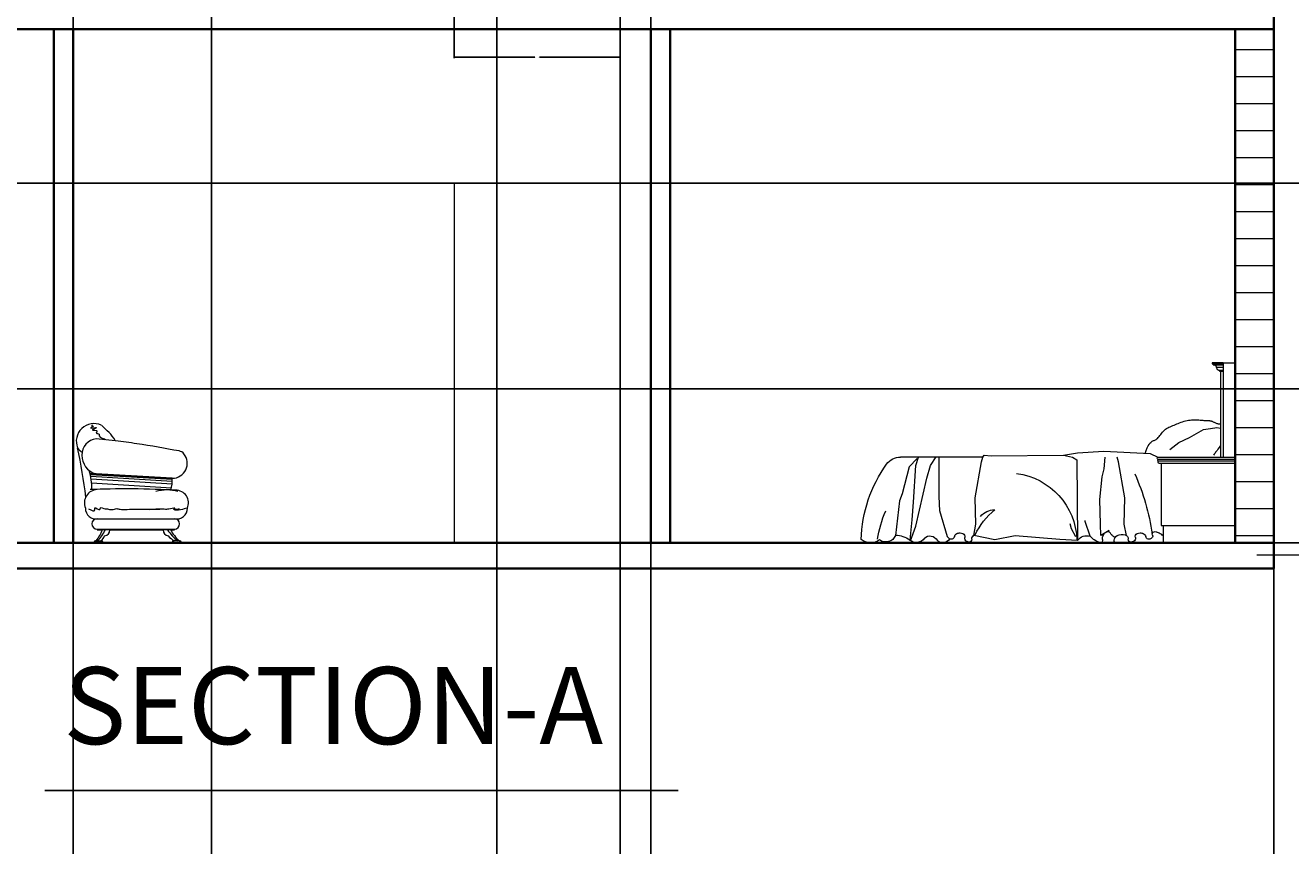
# Model space of a CAD drawing. Units: inches. Extents: x 1355 to 2746, y 1171 to 2751.
# Tile 21 of 24: x 2215 to 2510, y 2155 to 2346. Entities that reach past the tile are written whole.
import ezdxf

# ---------------------------------------------------------------- set-up
doc = ezdxf.new("R2010")
doc.units = ezdxf.units.IN
for name, color, linetype, lineweight in [('A-ANNO-DIMS', 2, 'Continuous', 18), ('A-ANNO-TEXT', 7, 'Continuous', 18), ('A-ANNO-TITL', 7, 'Continuous', 25), ('A-FURN', 8, 'Continuous', 13), ('A-SECT', 7, 'Continuous', 35), ('A-SECT-DOOR', 3, 'Continuous', 18), ('A-WALL-PATT', 252, 'Continuous', 13)]:
    doc.layers.add(name, color=color, linetype=linetype, lineweight=lineweight)
doc.styles.get("Standard").update_dxf_attribs({"font": 'arial.ttf'})
doc.dimstyles.get("Standard").update_dxf_attribs({"dimtxt": 0.18, "dimasz": 0.18, "dimexe": 0.18, "dimexo": 0.0625, "dimgap": 0.09, "dimtad": 0, "dimtih": 1, "dimtoh": 1, "dimdec": 4, "dimzin": 0, "dimdsep": 46, "dimtxsty": 'Standard', "dimcen": 0.09, "dimadec": 0, "dimazin": 0, "dimtfac": 1, "dimtdec": 4, "dimtofl": 0, "dimtmove": 0, "dimatfit": 3, "dimfxl": 1, "dimtolj": 1, "dimtzin": 0, "dimarcsym": 0})

# ---------------------------------------------------------------- blocks, each defined once
blk = doc.blocks.new('A$C2FF713C3')
for p, q in [((0, 1050.5), (0, 0.5)), ((70, 1050.5), (0, 1050.5)), ((70, 1050.5), (70, 500.5)), ((70, 1050.5), (133.7, 1050.5)), ((127.4, 1044.2), (70, 1044.2)), ((125.8, 1038), (70, 1038)), ((127.4, 1038), (125.8, 1038)), ((133.7, 1044.2), (127.4, 1044.2)), ((127.4, 1044.2), (127.4, 1038)), ((133.7, 1050.5), (133.7, 1044.2)), ((108.5, 1024.2), (70, 1024.2)), ((91.3, 1006.7), (70, 1006.7)), ((91.3, 1000.5), (70, 1000.5)), ((85, 1000.5), (85, 500.5)), ((97.5, 1006.7), (91.3, 1006.7)), ((91.3, 1006.7), (91.3, 1000.5)), ((87.4, 693.2), (83.6, 693.1)), ((107.4, 672.2), (85.3, 669.2)), ((91.2, 693.6), (87.4, 693.2)), ((95.1, 694.2), (91.2, 693.6)), ((99, 694.9), (95.1, 694.2)), ((102.9, 695.9), (99, 694.9)), ((106.8, 697), (102.9, 695.9)), ((110.7, 698.3), (106.8, 697)), ((144.4, 667.7), (107.4, 672.2)), ((114.5, 699.7), (110.7, 698.3)), ((118.2, 701.2), (114.5, 699.7)), ((121.8, 702.9), (118.2, 701.2)), ((125.3, 704.5), (121.8, 702.9)), ((128.7, 706.1), (125.3, 704.5)), ((131.9, 707.6), (128.7, 706.1)), ((134.9, 709), (131.9, 707.6)), ((137.8, 710.2), (134.9, 709)), ((140.5, 711.1), (137.8, 710.2)), ((143, 711.8), (140.5, 711.1)), ((145.5, 712.2), (143, 711.8)), ((184.4, 660.3), (144.4, 667.7)), ((148, 712.5), (145.5, 712.2)), ((150.6, 712.6), (148, 712.5)), ((153.6, 712.7), (150.6, 712.6)), ((156.9, 712.7), (153.6, 712.7)), ((160.7, 712.8), (156.9, 712.7)), ((165.1, 713), (160.7, 712.8)), ((170.2, 713.4), (165.1, 713)), ((175.9, 713.9), (170.2, 713.4)), ((182.3, 714.4), (175.9, 713.9)), ((189.2, 715), (182.3, 714.4)), ((196.5, 715.6), (189.2, 715)), ((204.1, 716.2), (196.5, 715.6)), ((212.1, 716.7), (204.1, 716.2)), ((220.3, 717.1), (212.1, 716.7)), ((228.7, 717.3), (220.3, 717.1)), ((237.2, 717.3), (228.7, 717.3)), ((245.8, 717.1), (237.2, 717.3)), ((254.4, 716.7), (245.8, 717.1)), ((263.2, 715.9), (254.4, 716.7)), ((271.9, 714.8), (263.2, 715.9)), ((280.7, 713.3), (271.9, 714.8)), ((289.5, 711.4), (280.7, 713.3)), ((298.2, 709.1), (289.5, 711.4)), ((306.9, 706.4), (298.2, 709.1)), ((315.5, 703.4), (306.9, 706.4)), ((324, 700.1), (315.5, 703.4)), ((332.3, 696.8), (324, 700.1)), ((340.6, 693.4), (332.3, 696.8)), ((348.7, 690), (340.6, 693.4)), ((356.6, 686.7), (348.7, 690)), ((364.3, 683.5), (356.6, 686.7)), ((371.9, 680.4), (364.3, 683.5)), ((379.2, 677.3), (371.9, 680.4)), ((386.3, 674), (379.2, 677.3)), ((393.1, 670.5), (386.3, 674)), ((399.8, 666.5), (393.1, 670.5)), ((406.2, 662.1), (399.8, 666.5)), ((267.2, 614.5), (184.4, 660.3)), ((327.9, 585), (267.2, 614.5)), ((412.3, 657), (406.2, 662.1)), ((418.1, 651.3), (412.3, 657)), ((423.7, 645.1), (418.1, 651.3)), ((429.1, 638.6), (423.7, 645.1)), ((434.2, 632), (429.1, 638.6)), ((439, 625.6), (434.2, 632)), ((443.7, 619.6), (439, 625.6)), ((448.1, 614.1), (443.7, 619.6)), ((452.4, 609.5), (448.1, 614.1)), ((456.4, 605.9), (452.4, 609.5)), ((460.3, 603), (456.4, 605.9)), ((464.2, 600.8), (460.3, 603)), ((468, 599.1), (464.2, 600.8)), ((471.7, 597.6), (468, 599.1)), ((475.6, 596.1), (471.7, 597.6)), ((479.6, 594.4), (475.6, 596.1)), ((483.7, 592.3), (479.6, 594.4)), ((488, 589.7), (483.7, 592.3)), ((84.9, 568), (93.7, 555.7)), ((93.7, 555.7), (100.6, 546.3)), ((100.6, 546.3), (105.9, 539)), ((105.9, 539), (110.1, 533.2)), ((110.1, 533.2), (113.9, 528.2)), ((113.9, 528.2), (117.6, 523.3)), ((117.6, 523.3), (121.8, 517.9)), ((121.8, 517.9), (127, 511.4)), ((381.3, 544.7), (327.9, 585)), ((495.7, 521.8), (450, 500.5)), ((492.6, 586), (488, 589.7)), ((497.4, 581), (492.6, 586)), ((766.6, 534.5), (495.7, 521.8)), ((502.4, 574.2), (497.4, 581)), ((507.8, 565.1), (502.4, 574.2)), ((513.4, 553.5), (507.8, 565.1)), ((519.3, 538.8), (513.4, 553.5)), ((525.6, 520.7), (519.3, 538.8)), ((919.2, 526), (766.6, 534.5)), ((1001, 512.1), (919.2, 526)), ((450, 500.5), (0, 500.5)), ((450, 488.5), (0, 488.5)), ((448.7, 477.5), (0, 477.5)), ((446.9, 465.5), (0, 465.5)), ((431.9, 465.5), (431.9, 100.5)), ((642.6, 263.3), (679.4, 472.9)), ((679.4, 472.9), (687.3, 500.5)), ((764.1, 432.4), (757.6, 500.5)), ((923, 485), (919.8, 13.9)), ((947.7, 499.8), (923, 485)), ((1001, 512.1), (947.7, 499.8)), ((1422.2, 508), (1001, 512.1)), ((1463.2, 511.6), (1422.2, 508)), ((1471.1, 500.5), (1463.2, 511.6)), ((1479, 472.9), (1471.1, 500.5)), ((1471.1, 500.5), (1951, 500.5)), ((1515.8, 263.3), (1479, 472.9)), ((1725.7, 369.9), (1725.7, 500.5)), ((1776.6, 450.8), (1743.5, 502.3)), ((1798.7, 377.3), (1776.6, 450.8)), ((1861.3, 450.8), (1846, 500.5)), ((1853.9, 491.3), (1901.8, 443.5)), ((1876, 237.5), (1861.3, 450.8)), ((1901.8, 443.5), (1942.3, 285.3)), ((775.1, 384.6), (764.1, 432.4)), ((789.8, 252.2), (775.1, 384.6)), ((1725.7, 270.6), (1725.7, 369.9)), ((1861.3, 97.8), (1798.7, 377.3)), ((646.3, 108.8), (642.6, 263.3)), ((786.1, 108.8), (789.8, 252.2)), ((1512.2, 108.8), (1515.8, 263.3)), ((1722, 186), (1725.7, 270.6)), ((1883.4, 134.6), (1876, 237.5)), ((1942.3, 285.3), (1957, 244.9)), ((1957, 244.9), (1981.3, 42.2)), ((1677.5, 36.3), (1722, 186)), ((431.9, 100.5), (0, 100.5)), ((419.9, 100.5), (419.9, 0.5)), ((634, 43.7), (646.3, 108.8)), ((782.5, 42.6), (786.1, 108.8)), ((844.9, 39.6), (874.4, 124.2)), ((874.4, 124.2), (875.1, 130)), ((956.4, 83.1), (931.8, 36.9)), ((964.4, 113.4), (956.4, 83.1)), ((1524.4, 43.7), (1512.2, 108.8)), ((1892.4, 12.1), (1861.3, 97.8)), ((1890.7, 57.3), (1883.4, 134.6)), ((0, 0.5), (419.9, 0.5)), ((734.6, 72), (782.5, 42.6)), ((919.8, 13.9), (1021.5, 19.4)), ((1021.5, 19.4), (1282.6, 41.6)), ((1282.6, 41.6), (1401.6, 17.8)), ((1401.6, 17.8), (1524.4, 43.7)), ((1894.7, 13.8), (1890.7, 57.3))]:
    blk.add_line(p, q)
for centre, radius, start, end in [((125, 1021.3), 16.8, 87.42116, 169.92904), ((90, 1023.7), 18.5, 293.7928, 1.50079), ((435.7, 473.3), 13.6, 324.97742, 17.95445), ((443.2, 483.7), 8.28, 310.99411, 35.0512), ((447.3, 494.5), 6.6, 294.61118, 65.38882), ((1951, 400.5), 100, 35.83195, 90), ((1396.7, 0.2), 783.8, 1.45705, 35.83195), ((1735.3, -117.1), 1261.8, 155.69024, 172.29016), ((1327.7, 3.6), 404.9, 97.57237, 178.02017), ((1400.1, 81.1), 112.5, 40.70885, 88.9264), ((1125.8, -139.2), 432.6, 25.56932, 50.29378), ((1449, -72.7), 642.9, 8.37443, 23.73381), ((259.9, 249), 261.9, 307.63119, 310.56693), ((478.1, -13.1), 79.2, 115.93806, 127.15402), ((517.4, -93.9), 169, 111.78143, 115.93806), ((474.5, 13.6), 53.3, 104.37799, 111.78143), ((466.1, 46.3), 19.5, 71.58245, 104.37799), ((464.6, 41.9), 24.2, 42.22901, 71.58245), ((490.7, 39.5), 10.2, 140.3102, 217.27929), ((475.7, 51.9), 9.23, 320.3102, 42.22901), ((513.6, 57), 39, 217.27929, 233.1579), ((500.7, 39.8), 17.5, 233.1579, 256.94088), ((500.6, 39.4), 17.2, 256.94088, 270), ((500.6, 74), 51.8, 270, 277.51528), ((505.3, 38.6), 16, 277.51528, 349.78267), ((546.4, 31.2), 25.7, 114.29273, 169.78267), ((554.4, 13.4), 45.2, 90, 114.29273), ((554.4, 20.7), 37.9, 63.42724, 90), ((562.2, 36.4), 20.3, 346.09021, 63.42724), ((601.7, 26.6), 20.3, 166.09021, 243.58133), ((609.7, 42.8), 38.3, 243.58133, 251.5824), ((612.4, 50.9), 46.9, 251.5824, 258.81111), ((606.5, 21.1), 16.5, 258.81111, 1.75785), ((648.9, 22.4), 25.9, 104.59371, 181.75785), ((658.8, -15.6), 65.2, 63.45814, 104.59371), ((673, 12.8), 33.4, 4.66977, 63.45814), ((674.1, 83.9), 58.7, 296.89415, 314.45228), ((713.3, 7.3), 7.4, 170.64836, 198.63453), ((677.4, 13.2), 29, 350.64836, 4.66977), ((711.6, 6.7), 5.58, 198.63453, 218.42959), ((207.6, 559.5), 724.9, 314.45228, 314.97091), ((575.9, 190.8), 203.8, 314.97091, 315.94905), ((696.8, 73.9), 35.6, 315.94905, 329.81727), ((762.4, 35.7), 40.4, 136.79901, 149.81727), ((740.9, 55.9), 10.9, 81.87802, 136.79901), ((738.1, 36.1), 30.8, 50.07733, 81.87802), ((735.6, 33.1), 34.7, 33.71681, 50.07733), ((690, 2.7), 89.5, 23.5428, 33.71681), ((747.6, 27.8), 26.6, 343.69737, 23.5428), ((788.5, 15.9), 15.9, 163.69737, 216.05798), ((783.9, 12.5), 10.2, 216.05798, 282.98191), ((759.3, 118.9), 119.4, 282.98191, 301.5385), ((783.2, 80.1), 73.8, 301.5385, 318.3377), ((782.8, 80.4), 74.3, 318.3377, 326.7067), ((863.8, -27), 69.2, 36.67542, 105.79154), ((957.7, 57), 57.3, 227.99499, 228.65775), ((1509.5, 22.4), 25.9, 358.24215, 61.16814), ((1551.9, 21.1), 16.5, 178.24215, 281.18889), ((1546, 50.9), 46.9, 281.18889, 288.4176), ((1548.7, 42.8), 38.3, 288.4176, 296.41867), ((1556.8, 26.6), 20.3, 296.41867, 13.90979), ((1596.2, 36.4), 20.3, 116.57276, 193.90979), ((1604, 20.7), 37.9, 90, 116.57276), ((1604, 13.4), 45.2, 65.70727, 90), ((1612, 31.2), 25.7, 10.21733, 65.70727), ((1653.1, 38.6), 16, 190.21733, 262.48472), ((1657.8, 74), 51.8, 262.48472, 270), ((1657.8, 39.4), 17.2, 270, 283.05912), ((1657.7, 39.8), 17.5, 283.05912, 306.8421), ((1704.6, 43.4), 43.5, 208.05971, 320.53056), ((1644.8, 57), 39, 306.8421, 322.72071), ((1667.7, 39.5), 10.2, 322.72071, 344.91412), ((1779.5, -6.4), 46.9, 46.72075, 151.78128), ((1859.7, 59.2), 57.3, 213.23769, 312.00501), ((1983.6, -94.9), 140.5, 91.35454, 127.50961), ((2036.9, 65.4), 60.1, 201.78863, 308.33048), ((2126, 84.9), 84.4, 232.07783, 309.92484)]:
    blk.add_arc(centre, radius, start, end)
blk = doc.blocks.new('A$C28ED0BDC')
for p, q in [((300.7, 778.6), (176.5, 792.9)), ((737.6, 490.8), (105.1, 529.1)), ((737.6, 485.8), (106.3, 524)), ((737.6, 480.8), (107.5, 518.9)), ((737.5, 465.8), (110.8, 503.7)), ((735.8, 445.9), (114.2, 483.5)), ((730.6, 416.3), (117.6, 453.3)), ((158.9, 100), (753.7, 100)), ((158.9, 100), (158.9, 95)), ((169.3, 180), (753.7, 180)), ((753.7, 100), (753.7, 95)), ((204.4, 0), (136.7, 0)), ((151.7, 10), (146, 10)), ((151.7, 10), (189.4, 10)), ((158.9, 95), (200.3, 95)), ((195, 10), (189.4, 10)), ((195, 10), (189.4, 10)), ((257.3, 95), (200.3, 95)), ((257.3, 95), (666.7, 95)), ((723.7, 95), (666.7, 95)), ((723.7, 95), (753.7, 95)), ((737.8, 0), (805.4, 0)), ((747.1, 10), (752.8, 10)), ((747.1, 10), (752.8, 10)), ((790.4, 10), (752.8, 10)), ((790.4, 10), (796.1, 10))]:
    blk.add_line(p, q)
for centre, radius, start, end in [((135.3, 776.3), 135.9, 65.3492, 202.21563), ((162.8, 673.6), 120, 83.43842, 170.98936), ((-3552.4, -58.3), 3647.1, 6.37823, 12.40155), ((93.2, 779.5), 99.8, 213.09621, 240.68048), ((193.2, 668.8), 150.8, 170.98936, 243.39142), ((780.2, 642.1), 60, 37.32442, 79.59851), ((737, 606.7), 115.8, 270.2622, 38.33495), ((-328, 418.8), 446.9, 358.17507, 17.23744), ((179.4, 641.3), 120, 243.39142, 252.67687), ((458.5, 479.3), 279.3, 343.50497, 2.36848), ((164.5, 301.2), 103.1, 93.095, 202.35798), ((696.5, 85.3), 315.8, 74.36238, 105.63762), ((763.8, 301.7), 98.3, 336.20857, 89.98148), ((151.5, 260.4), 82.4, 178.89673, 282.44534), ((771.4, 260.4), 82.4, 257.55466, 1.10327), ((158.9, 140), 40, 90, 270), ((753.7, 140), 40, 270, 90), ((148.9, -2), 12.3, 103.33506, 170.71519), ((-63.8, 189.5), 280.5, 320.20721, 340.30535), ((-29.3, 210.6), 277.5, 313.71744, 335.39036), ((124.1, 86.8), 100.8, 310.34673, 337.03101), ((192.2, -2), 12.3, 9.28481, 76.66494), ((210.9, 93.5), 46.4, 277.43329, 1.84553), ((713.1, 93.5), 46.4, 178.15447, 262.56671), ((987.3, 281.2), 341.5, 213.0378, 232.56776), ((831, 152.1), 162.1, 220.15958, 241.18286), ((1022.2, 260.8), 341.5, 209.04881, 227.25949), ((750, -2), 12.3, 103.33506, 170.71519), ((793.3, -2), 12.3, 9.28481, 76.66494)]:
    blk.add_arc(centre, radius, start, end)
for points, knots in [([(123.9, 901.3), (120.7, 897.9), (113.5, 890.1), (146.7, 895.3), (73.3, 866.1), (197.2, 892.5), (86.1, 854.7), (175.1, 866.1), (141.9, 832.2), (182.3, 838), (163.3, 800.3), (225.2, 796.2), (219.8, 787.9)], [0, 0, 0, 0, 9.765075, 22.239713, 47.817951, 93.447543, 130.976544, 169.416587, 185.180341, 209.428428, 221.888603, 276.469797, 276.469797, 276.469797, 276.469797]), ([(300.7, 778.6), (300.1, 779.6), (269.8, 832.3), (237.8, 855.2), (192, 899.8)], [244.920573, 244.920573, 244.920573, 244.920573, 247.928636, 395.738949, 395.738949, 395.738949, 395.738949]), ([(791, 701.1), (682.8, 721), (519.9, 750.6), (355.8, 771.9), (300.7, 778.6)], [18.761969, 18.761969, 18.761969, 18.761969, 348.756072, 515.290542, 515.290542, 515.290542, 515.290542]), ([(763.8, 400), (674.2, 404.2), (398.1, 413.1), (207.8, 407.5), (107.2, 404.2)], [0, 0, 0, 0, 269.198238, 571.026582, 571.026582, 571.026582, 571.026582]), ([(93.5, 256.7), (117.3, 244.2), (148.3, 227.9), (135.5, 280.6), (184.2, 233.2), (182.4, 277.4), (213.7, 254), (239, 258.5), (267.4, 245.2), (313.7, 262.9), (325.5, 247.1), (418.5, 255), (547.8, 252.8), (616.1, 255.7), (660.2, 256.5)], [0, 0, 0, 0, 49.407579, 64.565784, 105.844847, 118.345477, 155.269185, 167.410003, 198.361737, 241.285001, 308.128282, 447.747709, 520.592639, 652.828768, 652.828768, 652.828768, 652.828768]), ([(848.7, 261.5), (836.7, 257.2), (814, 248.9), (727, 241.4), (826.7, 263.1), (729.9, 243.1), (771.4, 265.6), (713.2, 252.2), (686.6, 252.2), (629, 252.7), (589.5, 250.5), (564.7, 249.2)], [0, 0, 0, 0, 49.380651, 92.855981, 126.791693, 168.915675, 179.762432, 213.696461, 251.182, 296.320949, 372.653556, 372.653556, 372.653556, 372.653556])]:
    blk.add_open_spline(points, degree=3, knots=knots)
blk = doc.blocks.new('DOOR-OPENING-SECTION')
for p, q in [((0, 84), (0, 0)), ((38.81, 84), (0, 84)), ((38.81, 84), (38.81, 0))]:
    blk.add_line(p, q)
blk = doc.blocks.new('*D94')
at = {"layer": 'A-ANNO-DIMS', "color": 0, "lineweight": -2, "transparency": 16777216}
for p, q in [((2314.9, 2351.34), (2314.9, 2338.62)), ((2353.71, 2351.34), (2353.71, 2338.62)), ((2315.08, 2338.8), (2333.78, 2338.8)), ((2353.53, 2338.8), (2334.83, 2338.8))]:
    blk.add_line(p, q, dxfattribs=at)
at = {"layer": 'A-ANNO-DIMS', "color": 0, "transparency": 16777216}
for points in [[(2315.08, 2338.83), (2315.08, 2338.77), (2314.9, 2338.8)], [(2353.53, 2338.83), (2353.53, 2338.77), (2353.71, 2338.8)]]:
    blk.add_solid(points, dxfattribs=at)
at = {"layer": 'Defpoints', "color": 0, "transparency": 16777216}
for p in [(2314.9, 2351.4), (2353.71, 2351.4), (2353.71, 2338.8)]:
    blk.add_point(p, dxfattribs=at)
at = {"layer": 'A-ANNO-DIMS', "color": 0, "transparency": 16777216, "insert": (2334.31, 2338.8), "char_height": 0.18, "attachment_point": 5}
blk.add_mtext('\\A1;39 TYP.', dxfattribs=at)
blk = doc.blocks.new('*D99')
at = {"layer": 'A-ANNO-DIMS', "color": 0, "lineweight": -2, "transparency": 16777216}
for p, q in [((2080.39, 2139.36), (2080.39, 2716.58)), ((2080.57, 2716.4), (2152.75, 2716.4)), ((2225.71, 2716.4), (2153.53, 2716.4)), ((2225.89, 2139.36), (2225.89, 2716.58))]:
    blk.add_line(p, q, dxfattribs=at)
at = {"layer": 'A-ANNO-DIMS', "color": 0, "transparency": 16777216}
for points in [[(2080.57, 2716.43), (2080.57, 2716.37), (2080.39, 2716.4)], [(2225.71, 2716.43), (2225.71, 2716.37), (2225.89, 2716.4)]]:
    blk.add_solid(points, dxfattribs=at)
at = {"layer": 'Defpoints', "color": 0, "transparency": 16777216}
for p in [(2225.89, 2716.4), (2080.39, 2139.3), (2225.89, 2139.3)]:
    blk.add_point(p, dxfattribs=at)
at = {"layer": 'A-ANNO-DIMS', "color": 0, "transparency": 16777216, "insert": (2153.14, 2716.4), "char_height": 0.18, "attachment_point": 5}
blk.add_mtext('\\A1;145.5', dxfattribs=at)
blk = doc.blocks.new('*D100')
at = {"layer": 'A-ANNO-DIMS', "color": 0, "lineweight": -2, "transparency": 16777216}
for p, q in [((2225.89, 2139.36), (2225.89, 2716.58)), ((2226.07, 2716.4), (2293.11, 2716.4)), ((2360.71, 2716.4), (2293.67, 2716.4)), ((2360.89, 2139.36), (2360.89, 2716.58))]:
    blk.add_line(p, q, dxfattribs=at)
at = {"layer": 'A-ANNO-DIMS', "color": 0, "transparency": 16777216}
for points in [[(2226.07, 2716.43), (2226.07, 2716.37), (2225.89, 2716.4)], [(2360.71, 2716.43), (2360.71, 2716.37), (2360.89, 2716.4)]]:
    blk.add_solid(points, dxfattribs=at)
at = {"layer": 'Defpoints', "color": 0, "transparency": 16777216}
for p in [(2360.89, 2716.4), (2225.89, 2139.3), (2360.89, 2139.3)]:
    blk.add_point(p, dxfattribs=at)
at = {"layer": 'A-ANNO-DIMS', "color": 0, "transparency": 16777216, "insert": (2293.39, 2716.4), "char_height": 0.18, "attachment_point": 5}
blk.add_mtext('\\A1;135', dxfattribs=at)
blk = doc.blocks.new('*D101')
at = {"layer": 'A-ANNO-DIMS', "color": 0, "lineweight": -2, "transparency": 16777216}
for p, q in [((2360.89, 2139.36), (2360.89, 2716.58)), ((2361.07, 2716.4), (2433.25, 2716.4)), ((2506.21, 2716.4), (2434.03, 2716.4)), ((2506.39, 2139.36), (2506.39, 2716.58))]:
    blk.add_line(p, q, dxfattribs=at)
at = {"layer": 'A-ANNO-DIMS', "color": 0, "transparency": 16777216}
for points in [[(2361.07, 2716.43), (2361.07, 2716.37), (2360.89, 2716.4)], [(2506.21, 2716.43), (2506.21, 2716.37), (2506.39, 2716.4)]]:
    blk.add_solid(points, dxfattribs=at)
at = {"layer": 'Defpoints', "color": 0, "transparency": 16777216}
for p in [(2506.39, 2716.4), (2360.89, 2139.3), (2506.39, 2139.3)]:
    blk.add_point(p, dxfattribs=at)
at = {"layer": 'A-ANNO-DIMS', "color": 0, "transparency": 16777216, "insert": (2433.64, 2716.4), "char_height": 0.18, "attachment_point": 5}
blk.add_mtext('\\A1;145.5', dxfattribs=at)
blk = doc.blocks.new('*D112')
at = {"layer": 'A-ANNO-DIMS', "color": 0, "lineweight": -2, "transparency": 16777216}
for p, q in [((2258.27, 2095.29), (2258.27, 2716.58)), ((2258.45, 2716.4), (2291.19, 2716.4)), ((2324.72, 2716.4), (2291.98, 2716.4)), ((2324.9, 2095.29), (2324.9, 2716.58))]:
    blk.add_line(p, q, dxfattribs=at)
at = {"layer": 'A-ANNO-DIMS', "color": 0, "transparency": 16777216}
for points in [[(2258.45, 2716.43), (2258.45, 2716.37), (2258.27, 2716.4)], [(2324.72, 2716.43), (2324.72, 2716.37), (2324.9, 2716.4)]]:
    blk.add_solid(points, dxfattribs=at)
at = {"layer": 'Defpoints', "color": 0, "transparency": 16777216}
for p in [(2324.9, 2716.4), (2258.27, 2095.22), (2324.9, 2095.22)]:
    blk.add_point(p, dxfattribs=at)
at = {"layer": 'A-ANNO-DIMS', "color": 0, "transparency": 16777216, "insert": (2291.58, 2716.4), "char_height": 0.18, "attachment_point": 5}
blk.add_mtext('\\A1;66.63', dxfattribs=at)
blk = doc.blocks.new('*D123')
at = {"layer": 'A-ANNO-DIMS', "color": 0, "lineweight": -2, "transparency": 16777216}
for p, q in [((1880.77, 2261.4), (2648.07, 2261.4)), ((2647.89, 2261.22), (2647.89, 2243.58)), ((2647.89, 2225.58), (2647.89, 2243.22)), ((1940.77, 2225.4), (2648.07, 2225.4))]:
    blk.add_line(p, q, dxfattribs=at)
at = {"layer": 'A-ANNO-DIMS', "color": 0, "transparency": 16777216}
for points in [[(2647.86, 2261.22), (2647.92, 2261.22), (2647.89, 2261.4)], [(2647.86, 2225.58), (2647.92, 2225.58), (2647.89, 2225.4)]]:
    blk.add_solid(points, dxfattribs=at)
at = {"layer": 'Defpoints', "color": 0, "transparency": 16777216}
for p in [(1880.71, 2261.4), (2647.89, 2261.4), (1940.71, 2225.4)]:
    blk.add_point(p, dxfattribs=at)
at = {"layer": 'A-ANNO-DIMS', "color": 0, "transparency": 16777216, "insert": (2647.89, 2243.4), "char_height": 0.18, "attachment_point": 5}
blk.add_mtext('\\A1;36', dxfattribs=at)
blk = doc.blocks.new('*D125')
at = {"layer": 'A-ANNO-DIMS', "color": 0, "lineweight": -2, "transparency": 16777216}
for p, q in [((1880.77, 2309.4), (2648.07, 2309.4)), ((2647.89, 2309.22), (2647.89, 2285.58)), ((2647.89, 2261.58), (2647.89, 2285.22)), ((1880.77, 2261.4), (2648.07, 2261.4))]:
    blk.add_line(p, q, dxfattribs=at)
at = {"layer": 'A-ANNO-DIMS', "color": 0, "transparency": 16777216}
for points in [[(2647.86, 2309.22), (2647.92, 2309.22), (2647.89, 2309.4)], [(2647.86, 2261.58), (2647.92, 2261.58), (2647.89, 2261.4)]]:
    blk.add_solid(points, dxfattribs=at)
at = {"layer": 'Defpoints', "color": 0, "transparency": 16777216}
for p in [(1880.71, 2309.4), (2647.89, 2309.4), (1880.71, 2261.4)]:
    blk.add_point(p, dxfattribs=at)
at = {"layer": 'A-ANNO-DIMS', "color": 0, "transparency": 16777216, "insert": (2647.89, 2285.4), "char_height": 0.18, "attachment_point": 5}
blk.add_mtext('\\A1;48', dxfattribs=at)
blk = doc.blocks.new('*D126')
at = {"layer": 'A-ANNO-DIMS', "color": 0, "lineweight": -2, "transparency": 16777216}
for p, q in [((2080.39, 2219.34), (2080.39, 1171.06)), ((2506.39, 2219.34), (2506.39, 1171.06)), ((2080.57, 1171.24), (2293.1, 1171.24)), ((2506.21, 1171.24), (2293.68, 1171.24))]:
    blk.add_line(p, q, dxfattribs=at)
at = {"layer": 'A-ANNO-DIMS', "color": 0, "transparency": 16777216}
for points in [[(2080.57, 1171.27), (2080.57, 1171.21), (2080.39, 1171.24)], [(2506.21, 1171.27), (2506.21, 1171.21), (2506.39, 1171.24)]]:
    blk.add_solid(points, dxfattribs=at)
at = {"layer": 'Defpoints', "color": 0, "transparency": 16777216}
for p in [(2080.39, 2219.4), (2506.39, 2219.4), (2506.39, 1171.24)]:
    blk.add_point(p, dxfattribs=at)
at = {"layer": 'A-ANNO-DIMS', "color": 0, "transparency": 16777216, "insert": (2293.39, 1171.24), "char_height": 0.18, "attachment_point": 5}
blk.add_mtext('\\A1;426', dxfattribs=at)
blk = doc.blocks.new('*D134')
at = {"layer": 'A-ANNO-DIMS', "color": 0, "lineweight": -2, "transparency": 16777216}
for p, q in [((2353.71, 2477.34), (2353.71, 1171.06)), ((2360.89, 2477.34), (2360.89, 1171.06)), ((2353.89, 1171.24), (2356.92, 1171.24)), ((2360.71, 1171.24), (2357.68, 1171.24))]:
    blk.add_line(p, q, dxfattribs=at)
at = {"layer": 'A-ANNO-DIMS', "color": 0, "transparency": 16777216}
for points in [[(2353.89, 1171.27), (2353.89, 1171.21), (2353.71, 1171.24)], [(2360.71, 1171.27), (2360.71, 1171.21), (2360.89, 1171.24)]]:
    blk.add_solid(points, dxfattribs=at)
at = {"layer": 'Defpoints', "color": 0, "transparency": 16777216}
for p in [(2353.71, 2477.4), (2360.89, 2477.4), (2360.89, 1171.24)]:
    blk.add_point(p, dxfattribs=at)
at = {"layer": 'A-ANNO-DIMS', "color": 0, "transparency": 16777216, "insert": (2357.3, 1171.24), "char_height": 0.18, "attachment_point": 5}
blk.add_mtext('\\A1;7.181', dxfattribs=at)

msp = doc.modelspace()

# ---------------------------------------------------------------- hatches: boundary and pattern name
at = {"layer": 'A-WALL-PATT'}
h = msp.add_hatch(dxfattribs=at)
h.set_pattern_fill('ANSI32', color=256)
h.paths.add_polyline_path([(1660.2083, 2139.3018), (1614.5977, 2139.3018), (1614.5977, 2130.3018), (1655.7083, 2130.3018), (1655.7083, 1981.8018), (1660.2083, 1981.8018), (1660.2083, 2090.7225), (1692.5832, 2090.7225), (1692.5832, 2095.2225), (1660.2083, 2095.2225)])
h.paths.add_polyline_path([(1523.7083, 2130.3018), (1554.5977, 2130.3018), (1554.5977, 2134.8018), (1554.5977, 2139.3018), (1514.7083, 2139.3018), (1514.7083, 2071.8385), (1523.7083, 2071.8385)])
h.paths.add_polyline_path([(1940.7083, 2139.3018), (1883.7928, 2139.3018), (1883.7928, 2130.3018), (1931.7083, 2130.3018), (1931.7083, 2098.3333), (1940.7083, 2098.3333)])
h.paths.add_polyline_path([(1799.7083, 2130.3018), (1823.7928, 2130.3018), (1823.7928, 2134.8018), (1823.7928, 2139.3018), (1795.2083, 2139.3018), (1795.2083, 2130.3018), (1795.2083, 2095.2225), (1759.2134, 2095.2225), (1759.2134, 2090.7225), (1795.2083, 2090.7225), (1795.2083, 1981.8018), (1799.7083, 1981.8018), (1799.7083, 1986.3018)])
h.paths.add_polyline_path([(1940.7083, 2038.3333), (1931.7083, 2038.3333), (1931.7083, 1986.3018), (1832.7083, 1986.3018), (1832.7083, 1947.1338), (1837.2083, 1947.1338), (1837.2083, 1981.8018), (1931.7083, 1981.8018), (1931.7083, 1967.1939), (1940.7083, 1967.1939)])
h.paths.add_polyline_path([(1940.7083, 1943.1939), (1931.7083, 1943.1939), (1931.7083, 1921.8018), (1837.2083, 1921.8018), (1837.2083, 1926.0511), (1832.7083, 1926.0511), (1832.7083, 1917.3018), (1931.7083, 1917.3018), (1931.7083, 1908.3321), (1940.7083, 1908.3321)])
h.paths.add_polyline_path([(1940.7083, 1884.3321), (1931.7083, 1884.3321), (1931.7083, 1869.3018), (1899.4583, 1869.3018), (1899.4583, 1864.8018), (1931.7083, 1864.8018), (1931.7083, 1773.3018), (1786.5143, 1773.3018), (1786.5143, 1764.3018), (1844.7083, 1764.3018), (1844.7083, 1748.9343), (1853.7083, 1748.9343), (1853.7083, 1764.3018), (1931.7083, 1764.3018), (1931.7083, 1652.9424), (1940.7083, 1652.9424)])
h.paths.add_polyline_path([(1799.7083, 1864.8018), (1806.0522, 1864.8018), (1806.0522, 1867.0518), (1806.0522, 1869.3018), (1799.7083, 1869.3018), (1799.7083, 1917.3018), (1799.7083, 1921.8018), (1795.2083, 1921.8018), (1795.2083, 1773.3018), (1799.7083, 1773.3018)])
h.paths.add_polyline_path([(1872.8988, 1867.0518), (1872.8988, 1869.3018), (1867.2083, 1869.3018), (1867.2083, 1917.3018), (1862.7083, 1917.3018), (1862.7083, 1869.3018), (1836.9546, 1869.3018), (1836.9546, 1864.8018), (1862.7083, 1864.8018), (1872.8988, 1864.8018)])
h.paths.add_polyline_path([(1749.2197, 1773.3018), (1655.7083, 1773.3018), (1523.7083, 1773.3018), (1523.7083, 1828.4963), (1514.7083, 1828.4963), (1514.7083, 1753.9033), (1519.2083, 1753.9033), (1523.7083, 1753.9033), (1523.7083, 1764.3018), (1655.7083, 1764.3018), (1749.2197, 1764.3018), (1749.2197, 1768.8018)])
h.paths.add_polyline_path([(1660.2083, 1921.8018), (1655.7083, 1921.8018), (1655.7083, 1917.3018), (1655.7083, 1773.3018), (1660.2083, 1773.3018)])
h.paths.add_polyline_path([(1523.7083, 2011.8385), (1514.7083, 2011.8385), (1514.7083, 1973.114), (1519.2083, 1973.114), (1523.7083, 1973.114), (1523.7083, 1976.8227), (1523.7083, 1981.8018), (1618.2083, 1981.8018), (1618.2083, 1921.8018), (1553.707, 1921.8018), (1553.707, 1917.3018), (1622.7083, 1917.3018), (1622.7083, 1919.5518), (1622.7083, 1921.8018), (1622.7083, 1986.3018), (1523.7083, 1986.3018)])
h.paths.add_polyline_path([(1529.6686, 1919.5518), (1529.6686, 1921.8018), (1523.7083, 1921.8018), (1523.7083, 1949.114), (1514.7083, 1949.114), (1514.7083, 1888.4963), (1523.7083, 1888.4963), (1523.7083, 1917.3018), (1529.6686, 1917.3018)])
h.paths.add_polyline_path([(1538.9419, 1775.643), (1585.5504, 1775.643), (1585.5504, 1798.0318), (1538.9419, 1798.0318)], flags=25)
h.paths.add_polyline_path([(1696.7097, 1497.3356), (1769.5651, 1497.3356), (1769.5651, 1523.4559), (1696.7097, 1523.4559)], flags=9)
h.paths.add_polyline_path([(1629.1643, 1230.5133), (1877.0879, 1230.5133), (1877.0879, 1267.606), (1629.1643, 1267.606)], flags=9)
h.paths.add_polyline_path([(2533.4462, 2215.4033), (2579.9292, 2215.4033), (2579.9292, 2231.889), (2533.4462, 2231.889)], flags=9)
h.paths.add_polyline_path([(2540.822, 2515.6945), (2594.2245, 2515.6945), (2594.2245, 2545.5463), (2540.822, 2545.5463)], flags=9)
h.paths.add_polyline_path([(2535.9857, 2588.2819), (2582.4687, 2588.2819), (2582.4687, 2604.7675), (2535.9857, 2604.7675)], flags=9)
h.paths.add_polyline_path([(2537.1627, 2617.1172), (2649.1245, 2617.1172), (2649.1245, 2633.6029), (2537.1627, 2633.6029)], flags=9)
h.paths.add_polyline_path([(2218.0051, 2168.228), (2363.9573, 2168.228), (2363.9573, 2205.3208), (2218.0051, 2205.3208)], flags=9)
h.paths.add_polyline_path([(1650.2156, 2165.3631), (1800.3547, 2165.3631), (1800.3547, 2202.4559), (1650.2156, 2202.4559)], flags=9)
h.paths.add_polyline_path([(2553.9592, 1610.7663), (2588.4203, 1610.7663), (2588.4203, 1660.2233), (2553.9592, 1660.2233)], flags=9)
h.paths.add_polyline_path([(1549.0868, 1648.2033), (1595.6952, 1648.2033), (1595.6952, 1670.5921), (1549.0868, 1670.5921)], flags=9)
h.paths.add_polyline_path([(1546.9525, 1502.0931), (1583.3413, 1502.0931), (1583.3413, 1524.4819), (1546.9525, 1524.4819)], flags=9)
h.paths.add_polyline_path([(1540.7704, 1433.4431), (1587.3788, 1433.4431), (1587.3788, 1455.8319), (1540.7704, 1455.8319)], flags=9)
h.paths.add_polyline_path([(1683.6524, 1321.5269), (1760.6169, 1321.5269), (1760.6169, 1333.8911), (1683.6524, 1333.8911)], flags=9)
h.paths.add_polyline_path([(1832.0485, 1356.0874), (1873.0989, 1356.0874), (1873.0989, 1378.4762), (1832.0485, 1378.4762)], flags=9)
h.paths.add_polyline_path([(1877.9694, 1431.2138), (1926.3827, 1431.2138), (1926.3827, 1453.578), (1877.9694, 1453.578)], flags=9)
h.paths.add_polyline_path([(1847.3106, 1499.8371), (1883.6994, 1499.8371), (1883.6994, 1522.2259), (1847.3106, 1522.2259)], flags=9)
h.paths.add_polyline_path([(1813.7015, 1640.7287), (1860.3099, 1640.7287), (1860.3099, 1663.1175), (1813.7015, 1663.1175)], flags=9)
h.paths.add_polyline_path([(1876.2576, 1710.2471), (1912.9452, 1710.2471), (1912.9452, 1732.6359), (1876.2576, 1732.6359)], flags=25)
h.paths.add_polyline_path([(1695.9163, 1715.3064), (1736.9668, 1715.3064), (1736.9668, 1737.6952), (1695.9163, 1737.6952)], flags=9)
h.paths.add_polyline_path([(1881.8583, 1888.9094), (1930.2717, 1888.9094), (1930.2717, 1911.2737), (1881.8583, 1911.2737)], flags=9)
h.paths.add_polyline_path([(1823.9298, 1798.6431), (1864.9803, 1798.6431), (1864.9803, 1821.0319), (1823.9298, 1821.0319)], flags=25)
h.paths.add_polyline_path([(1845.6062, 1948.1408), (1881.995, 1948.1408), (1881.995, 1970.5296), (1845.6062, 1970.5296)], flags=25)
h.paths.add_polyline_path([(1849.027, 1991.5151), (1895.6355, 1991.5151), (1895.6355, 2013.9039), (1849.027, 2013.9039)], flags=25)
h.paths.add_polyline_path([(1684.9725, 2113.8416), (1764.2658, 2113.8416), (1764.2658, 2126.2058), (1684.9725, 2126.2058)], flags=9)
h.paths.add_polyline_path([(1688.6193, 1913.0676), (1776.2005, 1913.0676), (1776.2005, 1935.4564), (1688.6193, 1935.4564)], flags=9)
h.paths.add_polyline_path([(1571.4689, 1930.9816), (1607.8577, 1930.9816), (1607.8577, 1953.3704), (1571.4689, 1953.3704)], flags=25)
h.paths.add_polyline_path([(1535.3581, 1998.3125), (1581.9665, 1998.3125), (1581.9665, 2020.7014), (1535.3581, 2020.7014)], flags=9)
h = msp.add_hatch(dxfattribs=at)
h.set_pattern_fill('ANSI32', color=256)
h.paths.add_polyline_path([(1749.2197, 1686.3018), (1732.6892, 1686.3018), (1523.7083, 1686.3018), (1523.7083, 1705.9033), (1514.7083, 1705.9033), (1514.7083, 1647.8732), (1519.2083, 1647.8732), (1523.7083, 1647.8732), (1523.7083, 1677.3018), (1655.7083, 1677.3018), (1655.7083, 1528.8018), (1660.2083, 1528.8018), (1660.2083, 1677.3018), (1732.6892, 1677.3018), (1749.2197, 1677.3018)])
h.paths.add_polyline_path([(1931.7083, 1686.3018), (1853.7083, 1686.3018), (1853.7083, 1703.5696), (1844.7083, 1703.5696), (1844.7083, 1686.3018), (1788.0274, 1686.3018), (1788.0274, 1677.3018), (1795.2083, 1677.3018), (1795.2083, 1528.8018), (1799.7083, 1528.8018), (1799.7083, 1677.3018), (1844.7083, 1677.3018), (1931.7083, 1677.3018)])
h.paths.add_polyline_path([(1931.7083, 1533.3018), (1844.7083, 1533.3018), (1832.7083, 1533.3018), (1832.7083, 1531.0518), (1832.7083, 1528.8018), (1832.7083, 1495.7519), (1837.2083, 1495.7519), (1837.2083, 1528.8018), (1931.7083, 1528.8018)])
h.paths.add_polyline_path([(1940.7083, 1592.9424), (1931.7083, 1592.9424), (1931.7083, 1506.7845), (1940.7083, 1506.7845)])
h.paths.add_polyline_path([(1940.7083, 1482.7845), (1936.2083, 1482.7845), (1931.7083, 1482.7845), (1931.7083, 1320.3018), (1880.7083, 1320.3018), (1880.7083, 1311.3018), (1940.7083, 1311.3018)])
h.paths.add_polyline_path([(1931.7083, 1468.8018), (1844.7083, 1468.8018), (1837.2083, 1468.8018), (1837.2083, 1474.34), (1832.7083, 1474.34), (1832.7083, 1468.8018), (1832.7083, 1464.3018), (1844.7083, 1464.3018), (1931.7083, 1464.3018)])
h.paths.add_polyline_path([(1863.8571, 1464.3018), (1859.3571, 1464.3018), (1859.3571, 1404.1662), (1838.1542, 1404.1662), (1838.1542, 1399.8018), (1869.4185, 1399.8018), (1869.4185, 1402.0518), (1869.4185, 1404.3018), (1863.8571, 1404.3018)])
h.paths.add_polyline_path([(1799.7083, 1399.6662), (1805.4082, 1399.6662), (1805.4082, 1401.9162), (1805.4082, 1404.1662), (1799.7083, 1404.1662), (1799.7083, 1464.3018), (1799.7083, 1468.8018), (1795.2083, 1468.8018), (1795.2083, 1356.2098), (1761.2597, 1356.2098), (1761.2597, 1351.7098), (1795.2083, 1351.7098), (1795.2083, 1320.3018), (1795.2083, 1311.3018), (1844.7083, 1311.3018), (1844.7083, 1315.8018), (1844.7083, 1320.3018), (1799.7083, 1320.3018)])
h.paths.add_polyline_path([(1692.9218, 1356.2098), (1660.2083, 1356.2098), (1660.2083, 1430.786), (1657.9583, 1430.786), (1655.7083, 1430.786), (1655.7083, 1320.3018), (1611.934, 1320.3018), (1611.934, 1311.3018), (1660.2083, 1311.3018), (1660.2083, 1351.7098), (1692.9218, 1351.7098)])
h.paths.add_polyline_path([(1523.7083, 1372.653), (1514.7083, 1372.653), (1514.7083, 1311.3018), (1551.934, 1311.3018), (1551.934, 1315.8018), (1551.934, 1320.3018), (1523.7083, 1320.3018)])
h.paths.add_polyline_path([(1523.7083, 1490.9023), (1514.7083, 1490.9023), (1514.7083, 1432.653), (1519.2083, 1432.653), (1523.7083, 1432.653)])
h.paths.add_polyline_path([(1660.2083, 1468.8018), (1622.7083, 1468.8018), (1622.7083, 1473.1566), (1618.2083, 1473.1566), (1618.2083, 1468.8018), (1523.7083, 1468.8018), (1523.7083, 1464.3018), (1655.7083, 1464.3018), (1655.7083, 1460.5634), (1660.2083, 1460.5634)])
h.paths.add_polyline_path([(1523.7083, 1587.8732), (1514.7083, 1587.8732), (1514.7083, 1514.9023), (1519.2083, 1514.9023), (1523.7083, 1514.9023)])
h.paths.add_polyline_path([(1622.7083, 1533.3018), (1523.7083, 1533.3018), (1523.7083, 1528.8018), (1618.2083, 1528.8018), (1618.2083, 1494.4205), (1622.7083, 1494.4205), (1622.7083, 1528.8018)])
h.paths.add_polyline_path([(1696.7097, 1497.3356), (1769.5651, 1497.3356), (1769.5651, 1523.4559), (1696.7097, 1523.4559)], flags=9)
h.paths.add_polyline_path([(1629.1643, 1230.5133), (1877.0879, 1230.5133), (1877.0879, 1267.606), (1629.1643, 1267.606)], flags=9)
h.paths.add_polyline_path([(2533.4462, 2215.4033), (2579.9292, 2215.4033), (2579.9292, 2231.889), (2533.4462, 2231.889)], flags=9)
h.paths.add_polyline_path([(2540.822, 2515.6945), (2594.2245, 2515.6945), (2594.2245, 2545.5463), (2540.822, 2545.5463)], flags=9)
h.paths.add_polyline_path([(2535.9857, 2588.2819), (2582.4687, 2588.2819), (2582.4687, 2604.7675), (2535.9857, 2604.7675)], flags=9)
h.paths.add_polyline_path([(2537.1627, 2617.1172), (2649.1245, 2617.1172), (2649.1245, 2633.6029), (2537.1627, 2633.6029)], flags=9)
h.paths.add_polyline_path([(2218.0051, 2168.228), (2363.9573, 2168.228), (2363.9573, 2205.3208), (2218.0051, 2205.3208)], flags=9)
h.paths.add_polyline_path([(1650.2156, 2165.3631), (1800.3547, 2165.3631), (1800.3547, 2202.4559), (1650.2156, 2202.4559)], flags=9)
h.paths.add_polyline_path([(2553.9592, 1610.7663), (2588.4203, 1610.7663), (2588.4203, 1660.2233), (2553.9592, 1660.2233)], flags=9)
h.paths.add_polyline_path([(1549.0868, 1648.2033), (1595.6952, 1648.2033), (1595.6952, 1670.5921), (1549.0868, 1670.5921)], flags=25)
h.paths.add_polyline_path([(1546.9525, 1502.0931), (1583.3413, 1502.0931), (1583.3413, 1524.4819), (1546.9525, 1524.4819)], flags=25)
h.paths.add_polyline_path([(1540.7704, 1433.4431), (1587.3788, 1433.4431), (1587.3788, 1455.8319), (1540.7704, 1455.8319)], flags=9)
h.paths.add_polyline_path([(1683.6524, 1321.5269), (1760.6169, 1321.5269), (1760.6169, 1333.8911), (1683.6524, 1333.8911)], flags=9)
h.paths.add_polyline_path([(1832.0485, 1356.0874), (1873.0989, 1356.0874), (1873.0989, 1378.4762), (1832.0485, 1378.4762)], flags=9)
h.paths.add_polyline_path([(1877.9694, 1431.2138), (1926.3827, 1431.2138), (1926.3827, 1453.578), (1877.9694, 1453.578)], flags=9)
h.paths.add_polyline_path([(1847.3106, 1499.8371), (1883.6994, 1499.8371), (1883.6994, 1522.2259), (1847.3106, 1522.2259)], flags=25)
h.paths.add_polyline_path([(1813.7015, 1640.7287), (1860.3099, 1640.7287), (1860.3099, 1663.1175), (1813.7015, 1663.1175)], flags=25)
h.paths.add_polyline_path([(1876.2576, 1710.2471), (1912.9452, 1710.2471), (1912.9452, 1732.6359), (1876.2576, 1732.6359)], flags=9)
h.paths.add_polyline_path([(1695.9163, 1715.3064), (1736.9668, 1715.3064), (1736.9668, 1737.6952), (1695.9163, 1737.6952)], flags=9)
h.paths.add_polyline_path([(1881.8583, 1888.9094), (1930.2717, 1888.9094), (1930.2717, 1911.2737), (1881.8583, 1911.2737)], flags=9)
h.paths.add_polyline_path([(1823.9298, 1798.6431), (1864.9803, 1798.6431), (1864.9803, 1821.0319), (1823.9298, 1821.0319)], flags=9)
h.paths.add_polyline_path([(1845.6062, 1948.1408), (1881.995, 1948.1408), (1881.995, 1970.5296), (1845.6062, 1970.5296)], flags=9)
h.paths.add_polyline_path([(1849.027, 1991.5151), (1895.6355, 1991.5151), (1895.6355, 2013.9039), (1849.027, 2013.9039)], flags=9)
h.paths.add_polyline_path([(1684.9725, 2113.8416), (1764.2658, 2113.8416), (1764.2658, 2126.2058), (1684.9725, 2126.2058)], flags=9)
h.paths.add_polyline_path([(1688.6193, 1913.0676), (1776.2005, 1913.0676), (1776.2005, 1935.4564), (1688.6193, 1935.4564)], flags=9)
h.paths.add_polyline_path([(1538.9419, 1775.643), (1585.5504, 1775.643), (1585.5504, 1798.0318), (1538.9419, 1798.0318)], flags=9)
h.paths.add_polyline_path([(1571.4689, 1930.9816), (1607.8577, 1930.9816), (1607.8577, 1953.3704), (1571.4689, 1953.3704)], flags=9)
h.paths.add_polyline_path([(1535.3581, 1998.3125), (1581.9665, 1998.3125), (1581.9665, 2020.7014), (1535.3581, 2020.7014)], flags=9)
h = msp.add_hatch(dxfattribs=at)
h.set_pattern_fill('ANSI31', color=256, scale=1.98709, angle=-45, style=0)
h.paths.add_polyline_path([(2497.3909, 2225.3999), (2506.3909, 2225.3999), (2506.3909, 2345.3999), (2497.3909, 2345.3999)])

# ---------------------------------------------------------------- linework, layer by layer
at = {"layer": 'A-ANNO-TEXT'}
msp.add_line((2502.4601, 2222.5737), (2530.0611, 2222.5737), dxfattribs=at)
at = {"layer": 'A-ANNO-TITL'}
msp.add_line((2219.3337, 2167.536), (2367.258, 2167.536), dxfattribs=at)
at = {"layer": 'A-SECT'}
for p, q in [((2506.3909, 2519.3999), (2506.3909, 2345.3999)), ((2506.3909, 2393.3999), (2506.3909, 2219.3999)), ((2506.3909, 2345.3999), (2080.3909, 2345.3999)), ((2221.3909, 2345.3999), (2221.3909, 2225.3999)), ((2225.8909, 2345.3999), (2225.8909, 2225.3999)), ((2360.8909, 2345.3999), (2360.8909, 2225.3999)), ((2365.3909, 2345.3999), (2365.3909, 2225.3999)), ((2497.3909, 2345.3999), (2497.3909, 2225.3999)), ((2506.3909, 2225.3999), (2080.3909, 2225.3999)), ((2506.3909, 2219.3999), (2080.3909, 2219.3999))]:
    msp.add_line(p, q, dxfattribs=at)

# ---------------------------------------------------------------- block references
at = {"layer": 'A-FURN'}
for name, p, xscale, yscale, zscale in [('A$C2FF713C3', (2497.3909, 2225.3801), -0.0400677785412672, 0.0400677785412672, 0.0400677785412672), ('A$C28ED0BDC', (2226.6669, 2225.5593), 0.0303702499100781, 0.0303702499100781, 0.0303702499100781)]:
    msp.add_blockref(name, p, dxfattribs=dict(at, xscale=xscale, yscale=yscale, zscale=zscale))
at = {"layer": 'A-SECT-DOOR'}
msp.add_blockref('DOOR-OPENING-SECTION', (2314.902, 2225.4), dxfattribs=at)

# ---------------------------------------------------------------- texts
at = {"layer": 'A-ANNO-TITL', "insert": (2223.6347, 2196.376), "char_height": 18, "attachment_point": 1}
msp.add_mtext_dynamic_manual_height_columns('SECTION-A', width=229.006142, gutter_width=12.5, heights=[0], dxfattribs=at)

# ---------------------------------------------------------------- dimensions: what is measured, and where the dimension line sits
at = {"layer": 'A-ANNO-DIMS'}
for base, p1, p2, override, picture, middle in [((2225.8909, 2716.3999), (2080.3909, 2139.3018), (2225.8909, 2139.3018), {"dimdec": 1, "dimlfac": 1, "dimrnd": 0, "dimzin": 0, "dimdsep": 46, "dimlunit": 2}, '*D99', (2153.1409, 2716.3999)), ((2360.8909, 2716.3999), (2225.8909, 2139.3018), (2360.8909, 2139.3018), {"dimdec": 0, "dimlfac": 1, "dimrnd": 0, "dimzin": 0, "dimdsep": 46, "dimlunit": 2}, '*D100', (2293.3909, 2716.3999)), ((2324.8959, 2716.3999), (2258.2658, 2095.2225), (2324.8959, 2095.2225), {"dimdec": 2, "dimlfac": 1, "dimrnd": 0, "dimzin": 0, "dimdsep": 46, "dimlunit": 2}, '*D112', (2291.5809, 2716.3999)), ((2506.3909, 2716.3999), (2360.8909, 2139.3018), (2506.3909, 2139.3018), {"dimdec": 1, "dimlfac": 1, "dimrnd": 0, "dimzin": 0, "dimdsep": 46, "dimlunit": 2}, '*D101', (2433.6409, 2716.3999)), ((2360.8909, 1171.2388), (2353.71, 2477.3999), (2360.8909, 2477.3999), {"dimdec": 3, "dimlfac": 1, "dimrnd": 0, "dimzin": 0, "dimdsep": 46, "dimlunit": 2}, '*D134', (2357.3004, 1171.2388)), ((2506.3909, 1171.2388), (2080.3909, 2219.3999), (2506.3909, 2219.3999), {"dimdec": 0, "dimlfac": 1, "dimrnd": 0, "dimzin": 0, "dimdsep": 46, "dimlunit": 2}, '*D126', (2293.3909, 1171.2388))]:
    dim = msp.add_linear_dim(base=base, p1=p1, p2=p2, dimstyle='Standard', override=override, dxfattribs=at)
    dim.commit()
    dim.dimension.update_dxf_attribs({"geometry": picture, "text_midpoint": middle})
dim = msp.add_linear_dim(base=(2353.71, 2338.7999), p1=(2314.9023, 2351.3999), p2=(2353.71, 2351.3999), text='<> TYP.', dimstyle='Standard', override={"dimdec": 0, "dimlfac": 1, "dimrnd": 0, "dimzin": 0, "dimdsep": 46, "dimlunit": 2}, dxfattribs=at)
dim.commit()
dim.dimension.update_dxf_attribs({"geometry": '*D94', "text_midpoint": (2334.3062, 2338.7999)})
for base, p1, p2, picture, middle in [((2647.886, 2309.3999), (1880.7083, 2261.3999), (1880.7083, 2309.3999), '*D125', (2647.886, 2285.3999)), ((2647.886, 2261.3999), (1940.7083, 2225.3999), (1880.7083, 2261.3999), '*D123', (2647.886, 2243.3999))]:
    dim = msp.add_linear_dim(base=base, p1=p1, p2=p2, angle=90, dimstyle='Standard', override={"dimdec": 0, "dimlfac": 1, "dimrnd": 0, "dimzin": 0, "dimdsep": 46, "dimlunit": 2}, dxfattribs=at)
    dim.commit()
    dim.dimension.update_dxf_attribs({"geometry": picture, "text_midpoint": middle})

doc.saveas('drawing.dxf')
